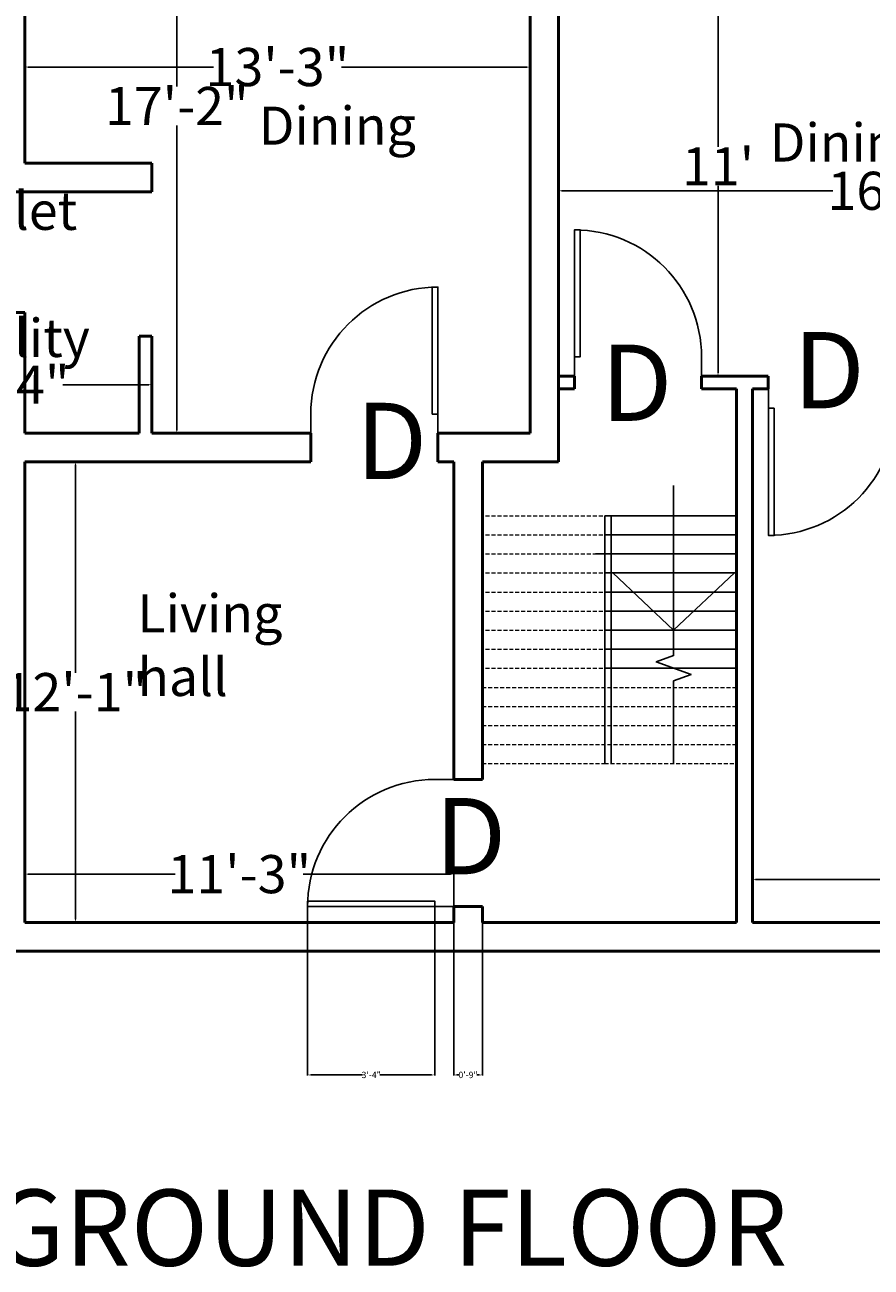
# Model space of a CAD drawing. Units: inches. Extents: x 409 to 7572, y 7 to 725.
# Tile 2 of 38: x 593 to 860, y 57 to 448. Entities that reach past the tile are written whole.
import ezdxf

# ---------------------------------------------------------------- set-up
doc = ezdxf.new("R2010")
doc.units = ezdxf.units.IN
doc.header["$MEASUREMENT"] = 0
doc.linetypes.add('HIDDEN', pattern=[0.375, 0.25, -0.125])
for name, color, linetype, lineweight in [('A-ANNO-DIMS', 2, 'Continuous', 18), ('A-ANNO-SYMB', 3, 'Continuous', 25), ('A-ANNO-TEXT', 7, 'Continuous', 35), ('A-AREA-IDEN', 7, 'Continuous', 25), ('A-DOOR', 3, 'Continuous', 25), ('A-FLOR-STRS', 6, 'Continuous', 25), ('A-FLOR-STRS-OVHD', 6, 'HIDDEN', 18), ('A-WALL', 7, 'Continuous', 50)]:
    doc.layers.add(name, color=color, linetype=linetype, lineweight=lineweight)
doc.styles.get("Standard").update_dxf_attribs({"font": 'arial.ttf'})
doc.dimstyles.get("Standard").update_dxf_attribs({"dimtxt": 2, "dimasz": 1, "dimexe": 0.18, "dimexo": 0.0625, "dimgap": 0.09, "dimtad": 0, "dimtih": 1, "dimtoh": 1, "dimdec": 0, "dimzin": 0, "dimdsep": 46, "dimlunit": 3, "dimtxsty": 'Standard', "dimcen": 0.09, "dimadec": 0, "dimazin": 0, "dimtfac": 1, "dimtdec": 0, "dimtofl": 0, "dimtmove": 0, "dimatfit": 3, "dimfxl": 1, "dimtolj": 1, "dimtzin": 0, "dimarcsym": 0})

# ---------------------------------------------------------------- blocks, each defined once
blk = doc.blocks.new('*U2')
for p, q in [((0, 0), (0, -6)), ((-40, 0), (-40, -6))]:
    blk.add_line(p, q)
blk.add_lwpolyline([(0, 0), (0, 40), (-1.75, 40), (-1.75, 0)], close=True)
blk.add_arc((0, 0), 40, 90, 180)
blk = doc.blocks.new('*U3')
for p, q in [((0, 0), (0, -6)), ((40, 0), (40, -6))]:
    blk.add_line(p, q)
blk.add_lwpolyline([(0, 0), (0, 40), (1.75, 40), (1.75, 0)], close=True)
blk.add_arc((0, 0), 40, 0, 90)
blk = doc.blocks.new('*U4')
for p, q in [((0, 0), (0, -6)), ((40, 0), (40, -6))]:
    blk.add_line(p, q)
blk.add_lwpolyline([(0, 0), (0, 40), (1.75, 40), (1.75, 0)], close=True)
blk.add_arc((0, 0), 40, 0, 90)
blk = doc.blocks.new('*U5')
for p, q in [((0, 0), (0, 6)), ((40, 0), (40, 6))]:
    blk.add_line(p, q)
blk.add_lwpolyline([(0, 0), (0, -40), (1.75, -40), (1.75, 0)], close=True)
blk.add_arc((0, 0), 40, 270, 0)
blk = doc.blocks.new('*D16')
at = {"layer": 'A-ANNO-DIMS', "color": 0, "lineweight": -2, "transparency": 16777216}
for p, q in [((822.16, 165.59), (822.16, 179.18)), ((823.16, 179), (870.02, 179)), ((957.16, 179), (910.29, 179)), ((958.16, 165.59), (958.16, 179.18))]:
    blk.add_line(p, q, dxfattribs=at)
at = {"layer": 'A-ANNO-DIMS', "color": 0, "transparency": 16777216}
for points in [[(823.16, 179.16), (823.16, 178.83), (822.16, 179)], [(957.16, 179.16), (957.16, 178.83), (958.16, 179)]]:
    blk.add_solid(points, dxfattribs=at)
at = {"layer": 'DEFPOINTS', "color": 0, "transparency": 16777216}
for p in [(958.16, 179), (822.16, 165.53), (958.16, 165.53)]:
    blk.add_point(p, dxfattribs=at)
at = {"layer": 'A-ANNO-DIMS', "color": 0, "transparency": 16777216, "insert": (890.16, 179), "char_height": 2, "attachment_point": 5}
blk.add_mtext('\\A1;{\\H6x;11\'-4"}', dxfattribs=at)
blk = doc.blocks.new('*D17')
at = {"layer": 'A-ANNO-DIMS', "color": 0, "lineweight": -2, "transparency": 16777216}
for p, q in [((593.16, 165.59), (593.16, 180.91)), ((594.16, 180.73), (640.52, 180.73)), ((727.16, 180.73), (680.79, 180.73)), ((728.16, 165.59), (728.16, 180.91))]:
    blk.add_line(p, q, dxfattribs=at)
at = {"layer": 'A-ANNO-DIMS', "color": 0, "transparency": 16777216}
for points in [[(594.16, 180.9), (594.16, 180.56), (593.16, 180.73)], [(727.16, 180.9), (727.16, 180.56), (728.16, 180.73)]]:
    blk.add_solid(points, dxfattribs=at)
at = {"layer": 'DEFPOINTS', "color": 0, "transparency": 16777216}
for p in [(728.16, 180.73), (593.16, 165.53), (728.16, 165.53)]:
    blk.add_point(p, dxfattribs=at)
at = {"layer": 'A-ANNO-DIMS', "color": 0, "transparency": 16777216, "insert": (660.66, 180.73), "char_height": 2, "attachment_point": 5}
blk.add_mtext('\\A1;{\\H6x;11\'-3"}', dxfattribs=at)
blk = doc.blocks.new('*D18')
at = {"layer": 'A-ANNO-DIMS', "color": 0, "lineweight": -2, "transparency": 16777216}
for p, q in [((593.22, 310.53), (609.26, 310.53)), ((609.08, 309.53), (609.08, 244.15)), ((609.08, 166.53), (609.08, 231.92)), ((593.22, 165.53), (609.26, 165.53))]:
    blk.add_line(p, q, dxfattribs=at)
at = {"layer": 'A-ANNO-DIMS', "color": 0, "transparency": 16777216}
for points in [[(608.91, 309.53), (609.25, 309.53), (609.08, 310.53)], [(608.91, 166.53), (609.25, 166.53), (609.08, 165.53)]]:
    blk.add_solid(points, dxfattribs=at)
at = {"layer": 'DEFPOINTS', "color": 0, "transparency": 16777216}
for p in [(593.16, 310.53), (593.16, 165.53), (609.08, 165.53)]:
    blk.add_point(p, dxfattribs=at)
at = {"layer": 'A-ANNO-DIMS', "color": 0, "transparency": 16777216, "insert": (609.08, 238.03), "char_height": 2, "attachment_point": 5}
blk.add_mtext('\\A1;{\\H6x;12\'-1"}', dxfattribs=at)
blk = doc.blocks.new('*D20')
at = {"layer": 'A-ANNO-DIMS', "color": 0, "lineweight": -2, "transparency": 16777216}
for p, q in [((593.16, 404.59), (593.16, 434.95)), ((594.16, 434.77), (652.52, 434.77)), ((751.16, 434.77), (692.79, 434.77)), ((752.16, 404.59), (752.16, 434.95))]:
    blk.add_line(p, q, dxfattribs=at)
at = {"layer": 'A-ANNO-DIMS', "color": 0, "transparency": 16777216}
for points in [[(594.16, 434.93), (594.16, 434.6), (593.16, 434.77)], [(751.16, 434.93), (751.16, 434.6), (752.16, 434.77)]]:
    blk.add_solid(points, dxfattribs=at)
at = {"layer": 'DEFPOINTS', "color": 0, "transparency": 16777216}
for p in [(752.16, 434.77), (593.16, 404.53), (752.16, 404.53)]:
    blk.add_point(p, dxfattribs=at)
at = {"layer": 'A-ANNO-DIMS', "color": 0, "transparency": 16777216, "insert": (672.66, 434.77), "char_height": 2, "attachment_point": 5}
blk.add_mtext('\\A1;{\\H6x;13\'-3"}', dxfattribs=at)
blk = doc.blocks.new('*D21')
at = {"layer": 'A-ANNO-DIMS', "color": 0, "lineweight": -2, "transparency": 16777216}
for p, q in [((650.09, 525.53), (640.81, 525.53)), ((640.99, 524.53), (640.99, 428.65)), ((640.99, 320.53), (640.99, 416.42)), ((658.09, 319.53), (640.81, 319.53))]:
    blk.add_line(p, q, dxfattribs=at)
at = {"layer": 'A-ANNO-DIMS', "color": 0, "transparency": 16777216}
for points in [[(640.83, 524.53), (641.16, 524.53), (640.99, 525.53)], [(640.83, 320.53), (641.16, 320.53), (640.99, 319.53)]]:
    blk.add_solid(points, dxfattribs=at)
at = {"layer": 'DEFPOINTS', "color": 0, "transparency": 16777216}
for p in [(650.16, 525.53), (640.99, 319.53), (658.16, 319.53)]:
    blk.add_point(p, dxfattribs=at)
at = {"layer": 'A-ANNO-DIMS', "color": 0, "transparency": 16777216, "insert": (640.99, 422.53), "char_height": 2, "attachment_point": 5}
blk.add_mtext('\\A1;{\\H6x;17\'-2"}', dxfattribs=at)
blk = doc.blocks.new('*D23')
at = {"layer": 'A-ANNO-DIMS', "color": 0, "lineweight": -2, "transparency": 16777216}
for p, q in [((761.16, 403.47), (761.16, 395.65)), ((953.16, 403.47), (953.16, 395.65)), ((762.16, 395.83), (847.45, 395.83)), ((952.16, 395.83), (866.86, 395.83))]:
    blk.add_line(p, q, dxfattribs=at)
at = {"layer": 'A-ANNO-DIMS', "color": 0, "transparency": 16777216}
for points in [[(762.16, 396), (762.16, 395.66), (761.16, 395.83)], [(952.16, 396), (952.16, 395.66), (953.16, 395.83)]]:
    blk.add_solid(points, dxfattribs=at)
at = {"layer": 'DEFPOINTS', "color": 0, "transparency": 16777216}
for p in [(761.16, 403.53), (953.16, 403.53), (953.16, 395.83)]:
    blk.add_point(p, dxfattribs=at)
at = {"layer": 'A-ANNO-DIMS', "color": 0, "transparency": 16777216, "insert": (857.16, 395.83), "char_height": 2, "attachment_point": 5}
blk.add_mtext("\\A1;{\\H6x;16'}", dxfattribs=at)
blk = doc.blocks.new('*D24')
at = {"layer": 'A-ANNO-DIMS', "color": 0, "lineweight": -2, "transparency": 16777216}
for p, q in [((815.42, 469.53), (811.17, 469.53)), ((811.35, 468.53), (811.35, 409.65)), ((811.35, 338.53), (811.35, 397.42)), ((816.59, 337.53), (811.17, 337.53))]:
    blk.add_line(p, q, dxfattribs=at)
at = {"layer": 'A-ANNO-DIMS', "color": 0, "transparency": 16777216}
for points in [[(811.19, 468.53), (811.52, 468.53), (811.35, 469.53)], [(811.19, 338.53), (811.52, 338.53), (811.35, 337.53)]]:
    blk.add_solid(points, dxfattribs=at)
at = {"layer": 'DEFPOINTS', "color": 0, "transparency": 16777216}
for p in [(815.48, 469.53), (811.35, 337.53), (816.66, 337.53)]:
    blk.add_point(p, dxfattribs=at)
at = {"layer": 'A-ANNO-DIMS', "color": 0, "transparency": 16777216, "insert": (811.35, 403.53), "char_height": 2, "attachment_point": 5}
blk.add_mtext("\\A1;{\\H6x;11'}", dxfattribs=at)
blk = doc.blocks.new('*D29')
at = {"layer": 'A-ANNO-DIMS', "color": 0, "lineweight": -2, "transparency": 16777216}
for p, q in [((545.16, 346.33), (545.16, 334.6)), ((633.16, 346.33), (633.16, 334.6)), ((546.16, 334.78), (573.17, 334.78)), ((632.16, 334.78), (605.15, 334.78))]:
    blk.add_line(p, q, dxfattribs=at)
at = {"layer": 'A-ANNO-DIMS', "color": 0, "transparency": 16777216}
for points in [[(546.16, 334.95), (546.16, 334.61), (545.16, 334.78)], [(632.16, 334.95), (632.16, 334.61), (633.16, 334.78)]]:
    blk.add_solid(points, dxfattribs=at)
at = {"layer": 'DEFPOINTS', "color": 0, "transparency": 16777216}
for p in [(545.16, 346.39), (633.16, 346.39), (633.16, 334.78)]:
    blk.add_point(p, dxfattribs=at)
at = {"layer": 'A-ANNO-DIMS', "color": 0, "transparency": 16777216, "insert": (589.16, 334.78), "char_height": 2, "attachment_point": 5}
blk.add_mtext('\\A1;{\\H6x;7\'-4"}', dxfattribs=at)
blk = doc.blocks.new('*D174')
at = {"layer": 'A-ANNO-DIMS', "color": 0, "lineweight": -2, "transparency": 16777216}
for p, q in [((728.16, 165.47), (728.16, 117.35)), ((737.16, 165.47), (737.16, 117.35)), ((729.16, 117.53), (729.91, 117.53)), ((736.16, 117.53), (735.4, 117.53))]:
    blk.add_line(p, q, dxfattribs=at)
at = {"layer": 'A-ANNO-DIMS', "color": 0, "transparency": 16777216}
for points in [[(729.16, 117.7), (729.16, 117.36), (728.16, 117.53)], [(736.16, 117.7), (736.16, 117.36), (737.16, 117.53)]]:
    blk.add_solid(points, dxfattribs=at)
at = {"layer": 'DEFPOINTS', "color": 0, "transparency": 16777216}
for p in [(728.16, 165.53), (737.16, 165.53), (737.16, 117.53)]:
    blk.add_point(p, dxfattribs=at)
at = {"layer": 'A-ANNO-DIMS', "color": 0, "transparency": 16777216, "insert": (732.66, 117.53), "char_height": 2, "attachment_point": 5}
blk.add_mtext('\\A1;0\'-9"', dxfattribs=at)
blk = doc.blocks.new('*D177')
at = {"layer": 'A-ANNO-DIMS', "color": 0, "lineweight": -2, "transparency": 16777216}
for p, q in [((682.16, 170.47), (682.16, 117.35)), ((722.16, 170.47), (722.16, 117.35)), ((683.16, 117.53), (699.41, 117.53)), ((721.16, 117.53), (704.9, 117.53))]:
    blk.add_line(p, q, dxfattribs=at)
at = {"layer": 'A-ANNO-DIMS', "color": 0, "transparency": 16777216}
for points in [[(683.16, 117.7), (683.16, 117.36), (682.16, 117.53)], [(721.16, 117.7), (721.16, 117.36), (722.16, 117.53)]]:
    blk.add_solid(points, dxfattribs=at)
at = {"layer": 'DEFPOINTS', "color": 0, "transparency": 16777216}
for p in [(682.16, 170.53), (722.16, 170.53), (722.16, 117.53)]:
    blk.add_point(p, dxfattribs=at)
at = {"layer": 'A-ANNO-DIMS', "color": 0, "transparency": 16777216, "insert": (702.16, 117.53), "char_height": 2, "attachment_point": 5}
blk.add_mtext('\\A1;3\'-4"', dxfattribs=at)

msp = doc.modelspace()

# ---------------------------------------------------------------- linework, layer by layer
at = {"layer": 'A-FLOR-STRS'}
for p, q in [((797.36, 303.06), (797.36, 257.53)), ((775.66, 293.53), (775.66, 215.53)), ((775.66, 293.53), (817.16, 293.53)), ((777.66, 293.53), (777.66, 215.53)), ((775.66, 287.53), (817.16, 287.53)), ((772.82, 281.53), (817.16, 281.53)), ((775.66, 275.53), (817.16, 275.53)), ((797.36, 257.53), (778.24, 275.53)), ((797.36, 257.53), (816.49, 275.53)), ((775.66, 269.53), (817.16, 269.53)), ((775.66, 263.53), (817.16, 263.53)), ((775.66, 257.53), (817.16, 257.53)), ((775.66, 251.53), (817.16, 251.53)), ((775.66, 245.53), (817.16, 245.53))]:
    msp.add_line(p, q, dxfattribs=at)
msp.add_lwpolyline([(797.36, 257.71), (797.36, 249.53), (791.87, 247.53), (802.86, 243.53), (797.36, 241.53), (797.36, 215.35)], dxfattribs=at)
at = {"layer": 'A-FLOR-STRS-OVHD', "ltscale": 5}
for p, q in [((738.16, 293.53), (775.66, 293.53)), ((738.16, 287.53), (775.66, 287.53)), ((738.16, 281.53), (772.82, 281.53)), ((738.16, 275.53), (775.66, 275.53)), ((738.16, 269.53), (775.66, 269.53)), ((738.16, 263.53), (775.66, 263.53)), ((738.16, 257.53), (775.66, 257.53)), ((738.16, 251.53), (775.66, 251.53)), ((738.16, 245.53), (775.66, 245.53)), ((737.16, 239.53), (817.16, 239.53)), ((737.16, 233.53), (817.16, 233.53)), ((737.16, 227.53), (817.16, 227.53)), ((737.16, 221.53), (817.16, 221.53)), ((737.16, 215.53), (775.66, 215.53)), ((775.66, 215.53), (817.16, 215.53))]:
    msp.add_line(p, q, dxfattribs=at)
at = {"layer": 'A-WALL'}
for p, q in [((593.16, 525.53), (593.16, 404.53)), ((752.16, 525.53), (752.16, 319.53)), ((761.16, 469.53), (761.16, 337.53)), ((633.16, 404.53), (593.16, 404.53)), ((633.16, 404.53), (633.16, 395.53)), ((593.16, 395.53), (545.16, 395.53)), ((633.16, 395.53), (593.16, 395.53)), ((593.16, 357.53), (584.16, 357.53)), ((593.16, 357.53), (593.16, 319.53)), ((633.16, 350.03), (629.16, 350.03)), ((629.16, 350.03), (629.16, 319.53)), ((633.16, 350.03), (633.16, 319.53)), ((761.16, 337.53), (766.16, 337.53)), ((761.16, 337.53), (761.16, 333.53)), ((766.16, 337.53), (766.16, 333.53)), ((806.16, 337.53), (827.16, 337.53)), ((806.16, 337.53), (806.16, 333.53)), ((827.16, 333.53), (827.16, 337.53)), ((761.16, 333.53), (766.16, 333.53)), ((761.16, 333.53), (761.16, 310.53)), ((806.16, 333.53), (817.16, 333.53)), ((817.16, 333.53), (817.16, 165.53)), ((822.16, 333.53), (822.16, 165.53)), ((822.16, 333.53), (827.16, 333.53)), ((629.16, 319.53), (593.16, 319.53)), ((683.16, 319.53), (633.16, 319.53)), ((683.16, 319.53), (683.16, 310.53)), ((752.16, 319.53), (723.16, 319.53)), ((723.16, 310.53), (723.16, 319.53)), ((593.16, 310.53), (593.16, 165.53)), ((683.16, 310.53), (593.16, 310.53)), ((728.16, 310.53), (723.16, 310.53)), ((728.16, 310.53), (728.16, 210.53)), ((761.16, 310.53), (737.16, 310.53)), ((737.16, 310.53), (737.16, 210.53)), ((728.16, 210.53), (737.16, 210.53)), ((737.16, 170.53), (728.16, 170.53)), ((728.16, 170.53), (728.16, 165.53)), ((737.16, 170.53), (737.16, 165.53)), ((593.16, 165.53), (728.16, 165.53)), ((737.16, 165.53), (817.16, 165.53)), ((822.16, 165.53), (958.16, 165.53)), ((584.16, 156.53), (958.16, 156.53))]:
    msp.add_line(p, q, dxfattribs=at)

# ---------------------------------------------------------------- block references
at = {"layer": 'A-DOOR'}
for name, p in [('*U4', (766.16, 343.53)), ('*U2', (723.16, 325.53)), ('*U5', (827.22, 327.37))]:
    msp.add_blockref(name, p, dxfattribs=at)
at = {"layer": 'A-DOOR', "rotation": 90}
msp.add_blockref('*U3', (722.16, 170.53), dxfattribs=at)

# ---------------------------------------------------------------- texts
at = {"layer": 'A-ANNO-SYMB', "char_height": 24, "attachment_point": 1}
for insert in [(834.99, 351.37), (774.45, 347.4), (697.29, 329.09), (722.16, 204.69)]:
    msp.add_mtext_dynamic_manual_height_columns('D', width=19.1972, gutter_width=1, heights=[0], dxfattribs=dict(at, insert=insert))
at = {"layer": 'A-ANNO-TEXT', "insert": (583.19, 81.45), "char_height": 24, "attachment_point": 1}
msp.add_mtext_dynamic_manual_height_columns('GROUND FLOOR', width=577.2242, gutter_width=1, heights=[0], dxfattribs=at)
at = {"layer": 'A-AREA-IDEN', "char_height": 12, "attachment_point": 1}
for s, width, insert in [('Dining ', 67.5069, (666.76, 422.33)), ('Dining ', 67.5069, (827.59, 417.03)), ('toilet / utility', 49.2946, (569.16, 395.53)), ('Living hall', 58.8843, (628.58, 268.81))]:
    msp.add_mtext_dynamic_manual_height_columns(s, width=width, gutter_width=1, heights=[0], dxfattribs=dict(at, insert=insert))

# ---------------------------------------------------------------- dimensions: what is measured, and where the dimension line sits
at = {"layer": 'A-ANNO-DIMS'}
dim = msp.add_linear_dim(base=(640.99, 319.53), p1=(650.16, 525.53), p2=(658.16, 319.53), angle=90, text='{\\H6x;<>}', dimstyle='Standard', override={"dimclrd": 0, "dimclre": 0, "dimclrt": 0}, dxfattribs=at)
dim.commit()
dim.dimension.update_dxf_attribs({"geometry": '*D21', "text_midpoint": (640.99, 422.53), "dimtype": 160})
for base, p1, p2, picture, middle in [((811.35, 337.53), (815.48, 469.53), (816.66, 337.53), '*D24', (811.35, 403.53)), ((609.08, 165.53), (593.16, 310.53), (593.16, 165.53), '*D18', (609.08, 238.03))]:
    dim = msp.add_linear_dim(base=base, p1=p1, p2=p2, angle=90, text='{\\H6x;<>}', dimstyle='Standard', override={"dimclrd": 0, "dimclre": 0, "dimclrt": 0}, dxfattribs=at)
    dim.commit()
    dim.dimension.update_dxf_attribs({"geometry": picture, "text_midpoint": middle})
for base, p1, p2, picture, middle in [((752.16, 434.77), (593.16, 404.53), (752.16, 404.53), '*D20', (672.66, 434.77)), ((633.16, 334.78), (545.16, 346.39), (633.16, 346.39), '*D29', (589.16, 334.78)), ((728.16, 180.73), (593.16, 165.53), (728.16, 165.53), '*D17', (660.66, 180.73)), ((958.16, 179), (822.16, 165.53), (958.16, 165.53), '*D16', (890.16, 179))]:
    dim = msp.add_linear_dim(base=base, p1=p1, p2=p2, text='{\\H6x;<>}', dimstyle='Standard', override={"dimclrd": 0, "dimclre": 0, "dimclrt": 0}, dxfattribs=at)
    dim.commit()
    dim.dimension.update_dxf_attribs({"geometry": picture, "text_midpoint": middle})
dim = msp.add_linear_dim(base=(953.16, 395.83), p1=(761.16, 403.53), p2=(953.16, 403.53), text='{\\H6x;<>}', dimstyle='Standard', override={"dimclrd": 0, "dimclre": 0, "dimclrt": 0}, dxfattribs=at)
dim.commit()
dim.dimension.update_dxf_attribs({"geometry": '*D23', "text_midpoint": (857.16, 395.83), "dimtype": 160})
for base, p1, p2, picture, middle in [((722.16, 117.53), (682.16, 170.53), (722.16, 170.53), '*D177', (702.16, 117.53)), ((737.16, 117.53), (728.16, 165.53), (737.16, 165.53), '*D174', (732.66, 117.53))]:
    dim = msp.add_linear_dim(base=base, p1=p1, p2=p2, dimstyle='Standard', override={"dimdec": 1, "dimlfac": 1, "dimrnd": 0, "dimzin": 1, "dimdsep": 46, "dimlunit": 4, "dimfrac": 2}, dxfattribs=at)
    dim.commit()
    dim.dimension.update_dxf_attribs({"geometry": picture, "text_midpoint": middle})

doc.saveas('drawing.dxf')
